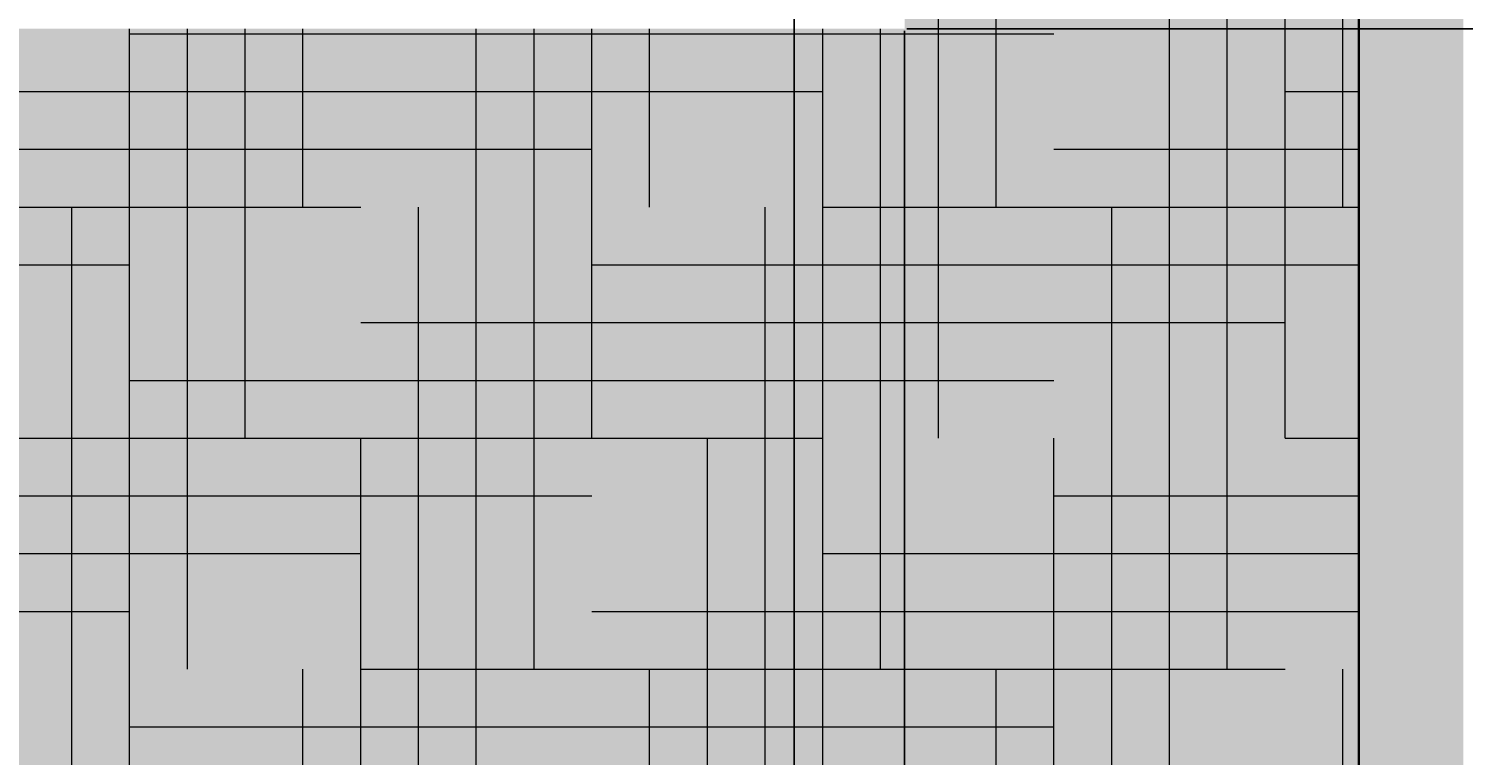
# Model space of a CAD drawing. Units: feet. Extents: x 2695 to 2912, y 795 to 1139.
# Tile 9 of 83: x 2734 to 2774, y 855 to 875. Entities that reach past the tile are written whole.
import ezdxf

# ---------------------------------------------------------------- set-up
doc = ezdxf.new("R2010")
doc.units = ezdxf.units.FT
for name, color, linetype, lineweight in [('A-ANNO-DIMS', 2, 'Continuous', 18), ('A-ELEV', 7, 'Continuous', 35), ('A-ELEV-PATT', 252, 'Continuous', 13)]:
    doc.layers.add(name, color=color, linetype=linetype, lineweight=lineweight)
doc.styles.get("Standard").update_dxf_attribs({"font": 'arial.ttf'})
doc.dimstyles.get("Standard").update_dxf_attribs({"dimtxt": 0.18, "dimasz": 0.18, "dimexe": 0.18, "dimexo": 0.0625, "dimgap": 0.09, "dimtad": 0, "dimtih": 1, "dimtoh": 1, "dimdec": 1, "dimzin": 0, "dimdsep": 46, "dimlunit": 3, "dimtxsty": 'Standard', "dimcen": 0.09, "dimadec": 0, "dimazin": 0, "dimtfac": 1, "dimtdec": 1, "dimtofl": 0, "dimtmove": 0, "dimatfit": 3, "dimfxl": 1, "dimtolj": 1, "dimtzin": 0, "dimarcsym": 0})

# ---------------------------------------------------------------- blocks, each defined once
blk = doc.blocks.new('*D3')
at = {"layer": 'A-ANNO-DIMS', "color": 0, "lineweight": -2, "transparency": 16777216}
for p, q in [((2724.189, 874.795), (2724.189, 794.976)), ((2758.151, 874.795), (2758.151, 794.976)), ((2724.369, 795.156), (2740.777, 795.156)), ((2757.971, 795.156), (2741.564, 795.156))]:
    blk.add_line(p, q, dxfattribs=at)
at = {"layer": 'A-ANNO-DIMS', "color": 0, "transparency": 16777216}
for points in [[(2724.369, 795.186), (2724.369, 795.126), (2724.189, 795.156)], [(2757.971, 795.186), (2757.971, 795.126), (2758.151, 795.156)]]:
    blk.add_solid(points, dxfattribs=at)
at = {"layer": 'Defpoints', "color": 0, "transparency": 16777216}
for p in [(2724.189, 874.857), (2758.151, 874.857), (2758.151, 795.156)]:
    blk.add_point(p, dxfattribs=at)
at = {"layer": 'A-ANNO-DIMS', "color": 0, "transparency": 16777216, "insert": (2741.17, 795.156), "char_height": 0.18, "attachment_point": 5}
blk.add_mtext('\\A1;33.96', dxfattribs=at)
blk = doc.blocks.new('*D4')
at = {"layer": 'A-ANNO-DIMS', "color": 0, "lineweight": -2, "transparency": 16777216}
for p, q in [((2758.151, 874.795), (2758.151, 794.976)), ((2773.503, 810.868), (2773.503, 794.976)), ((2758.331, 795.156), (2765.441, 795.156)), ((2773.323, 795.156), (2766.213, 795.156))]:
    blk.add_line(p, q, dxfattribs=at)
at = {"layer": 'A-ANNO-DIMS', "color": 0, "transparency": 16777216}
for points in [[(2758.331, 795.186), (2758.331, 795.126), (2758.151, 795.156)], [(2773.323, 795.186), (2773.323, 795.126), (2773.503, 795.156)]]:
    blk.add_solid(points, dxfattribs=at)
at = {"layer": 'Defpoints', "color": 0, "transparency": 16777216}
for p in [(2758.151, 874.857), (2773.503, 810.931), (2773.503, 795.156)]:
    blk.add_point(p, dxfattribs=at)
at = {"layer": 'A-ANNO-DIMS', "color": 0, "transparency": 16777216, "insert": (2765.827, 795.156), "char_height": 0.18, "attachment_point": 5}
blk.add_mtext('\\A1;15.35', dxfattribs=at)
blk = doc.blocks.new('*D13')
at = {"layer": 'A-ANNO-DIMS', "color": 0, "lineweight": -2, "transparency": 16777216}
for p, q in [((2758.214, 874.857), (2911.424, 874.857)), ((2911.244, 874.677), (2911.244, 843.076)), ((2911.244, 811.111), (2911.244, 842.712)), ((2890.699, 810.931), (2911.424, 810.931))]:
    blk.add_line(p, q, dxfattribs=at)
at = {"layer": 'A-ANNO-DIMS', "color": 0, "transparency": 16777216}
for points in [[(2911.214, 874.677), (2911.274, 874.677), (2911.244, 874.857)], [(2911.214, 811.111), (2911.274, 811.111), (2911.244, 810.931)]]:
    blk.add_solid(points, dxfattribs=at)
at = {"layer": 'Defpoints', "color": 0, "transparency": 16777216}
for p in [(2758.151, 874.857), (2911.244, 874.857), (2890.636, 810.931)]:
    blk.add_point(p, dxfattribs=at)
at = {"layer": 'A-ANNO-DIMS', "color": 0, "transparency": 16777216, "insert": (2911.244, 842.894), "char_height": 0.18, "attachment_point": 5}
blk.add_mtext('\\A1;63.93', dxfattribs=at)
blk = doc.blocks.new('*D14')
at = {"layer": 'A-ANNO-DIMS', "color": 0, "lineweight": -2, "transparency": 16777216}
for p, q in [((2838.439, 905.514), (2911.424, 905.514)), ((2911.244, 905.334), (2911.244, 890.368)), ((2911.244, 875.037), (2911.244, 890.004)), ((2758.214, 874.857), (2911.424, 874.857))]:
    blk.add_line(p, q, dxfattribs=at)
at = {"layer": 'A-ANNO-DIMS', "color": 0, "transparency": 16777216}
for points in [[(2911.214, 905.334), (2911.274, 905.334), (2911.244, 905.514)], [(2911.214, 875.037), (2911.274, 875.037), (2911.244, 874.857)]]:
    blk.add_solid(points, dxfattribs=at)
at = {"layer": 'Defpoints', "color": 0, "transparency": 16777216}
for p in [(2838.377, 905.514), (2911.244, 905.514), (2758.151, 874.857)]:
    blk.add_point(p, dxfattribs=at)
at = {"layer": 'A-ANNO-DIMS', "color": 0, "transparency": 16777216, "insert": (2911.244, 890.186), "char_height": 0.18, "attachment_point": 5}
blk.add_mtext('\\A1;30.66', dxfattribs=at)
blk = doc.blocks.new('*D24')
at = {"layer": 'A-ANNO-DIMS', "color": 0, "lineweight": -2, "transparency": 16777216}
for p, q in [((2730.708, 936.868), (2730.708, 794.976)), ((2755.112, 936.868), (2755.112, 794.976)), ((2730.888, 795.156), (2742.446, 795.156)), ((2754.932, 795.156), (2743.375, 795.156))]:
    blk.add_line(p, q, dxfattribs=at)
at = {"layer": 'A-ANNO-DIMS', "color": 0, "transparency": 16777216}
for points in [[(2730.888, 795.186), (2730.888, 795.126), (2730.708, 795.156)], [(2754.932, 795.186), (2754.932, 795.126), (2755.112, 795.156)]]:
    blk.add_solid(points, dxfattribs=at)
at = {"layer": 'Defpoints', "color": 0, "transparency": 16777216}
for p in [(2730.708, 936.931), (2755.112, 936.931), (2755.112, 795.156)]:
    blk.add_point(p, dxfattribs=at)
at = {"layer": 'A-ANNO-DIMS', "color": 0, "transparency": 16777216, "insert": (2742.91, 795.156), "char_height": 0.18, "attachment_point": 5}
blk.add_mtext('\\A1;24.404', dxfattribs=at)
blk = doc.blocks.new('*D25')
at = {"layer": 'A-ANNO-DIMS', "color": 0, "lineweight": -2, "transparency": 16777216}
for p, q in [((2755.112, 936.868), (2755.112, 794.976)), ((2770.636, 936.868), (2770.636, 794.976)), ((2755.292, 795.156), (2762.419, 795.156)), ((2770.456, 795.156), (2763.329, 795.156))]:
    blk.add_line(p, q, dxfattribs=at)
at = {"layer": 'A-ANNO-DIMS', "color": 0, "transparency": 16777216}
for points in [[(2755.292, 795.186), (2755.292, 795.126), (2755.112, 795.156)], [(2770.456, 795.186), (2770.456, 795.126), (2770.636, 795.156)]]:
    blk.add_solid(points, dxfattribs=at)
at = {"layer": 'Defpoints', "color": 0, "transparency": 16777216}
for p in [(2755.112, 936.931), (2770.636, 936.931), (2770.636, 795.156)]:
    blk.add_point(p, dxfattribs=at)
at = {"layer": 'A-ANNO-DIMS', "color": 0, "transparency": 16777216, "insert": (2762.874, 795.156), "char_height": 0.18, "attachment_point": 5}
blk.add_mtext('\\A1;15.524', dxfattribs=at)

msp = doc.modelspace()

# ---------------------------------------------------------------- hatches: boundary and pattern name
at = {"layer": 'A-ELEV-PATT'}
h = msp.add_hatch(color=256, dxfattribs=at)
h.set_gradient(color1=(147, 149, 152), color2=(147, 149, 152), tint=1)
h.paths.add_polyline_path([(2770.6361, 1118.4096), (2710.6361, 1118.4096), (2710.6361, 1062.9306), (2770.6361, 1062.9306)])
h.paths.add_polyline_path([(2890.6361, 1103.3378), (2770.6361, 1103.3378), (2770.6361, 1062.9306), (2890.6361, 1062.9306)])
h.paths.add_polyline_path([(2730.7081, 1048.1052), (2755.1125, 1048.1052), (2755.1125, 936.9306), (2770.6361, 936.9306), (2770.6361, 1050.3105), (2715.8852, 1050.3105), (2715.8852, 936.9306), (2730.7081, 936.9306)])
h.paths.add_polyline_path([(2890.6361, 1050.3105), (2770.6361, 1050.3105), (2770.6361, 971.9673), (2778.0341, 971.9673), (2778.0341, 1020.8235), (2843.575, 1020.8235), (2843.575, 971.9673), (2890.6361, 971.9673)])
h.paths.add_polyline_path([(2888.1882, 970.7156), (2843.575, 970.7156), (2843.575, 964.8267), (2888.1882, 964.8267)])
h.paths.add_polyline_path([(2888.1882, 964.1328), (2843.575, 964.1328), (2843.575, 956.614), (2888.1882, 956.614)])
h.paths.add_polyline_path([(2888.1882, 955.9202), (2843.575, 955.9202), (2843.575, 949.2892), (2888.1882, 949.2892)])
h.paths.add_polyline_path([(2888.1882, 948.5954), (2843.575, 948.5954), (2843.575, 941.3507), (2888.1882, 941.3507)])
h.paths.add_polyline_path([(2888.1882, 940.6569), (2843.575, 940.6569), (2843.575, 936.9306), (2888.1882, 936.9306)])
h.paths.add_polyline_path([(2890.6361, 970.7156), (2888.9368, 970.7156), (2888.9368, 964.8267), (2890.6361, 964.8267)])
h.paths.add_polyline_path([(2890.6361, 964.1328), (2888.9368, 964.1328), (2888.9368, 956.614), (2890.6361, 956.614)])
h.paths.add_polyline_path([(2890.6361, 955.9202), (2888.9368, 955.9202), (2888.9368, 949.2892), (2890.6361, 949.2892)])
h.paths.add_polyline_path([(2890.6361, 940.6569), (2888.9368, 940.6569), (2888.9368, 936.9306), (2890.6361, 936.9306)])
h.paths.add_polyline_path([(2890.6361, 948.5954), (2888.9368, 948.5954), (2888.9368, 941.3507), (2890.6361, 941.3507)])
h.paths.add_polyline_path([(2772.5216, 970.7156), (2770.6361, 970.7156), (2770.6361, 964.8267), (2772.5216, 964.8267)])
h.paths.add_polyline_path([(2772.5216, 964.1328), (2770.6361, 964.1328), (2770.6361, 956.614), (2772.5216, 956.614)])
h.paths.add_polyline_path([(2772.5216, 955.9202), (2770.6361, 955.9202), (2770.6361, 949.2892), (2772.5216, 949.2892)])
h.paths.add_polyline_path([(2772.5216, 948.5954), (2770.6361, 948.5954), (2770.6361, 941.3507), (2772.5216, 941.3507)])
h.paths.add_polyline_path([(2772.5216, 940.6569), (2770.6361, 940.6569), (2770.6361, 936.9306), (2772.5216, 936.9306)])
h.paths.add_polyline_path([(2778.0341, 940.6569), (2773.2702, 940.6569), (2773.2702, 936.9306), (2778.0341, 936.9306)])
h.paths.add_polyline_path([(2778.0341, 970.7156), (2773.2702, 970.7156), (2773.2702, 964.8267), (2778.0341, 964.8267)])
h.paths.add_polyline_path([(2778.0341, 964.1328), (2773.2702, 964.1328), (2773.2702, 956.614), (2778.0341, 956.614)])
h.paths.add_polyline_path([(2778.0341, 955.9202), (2773.2702, 955.9202), (2773.2702, 949.2892), (2778.0341, 949.2892)])
h.paths.add_polyline_path([(2778.0341, 948.5954), (2773.2702, 948.5954), (2773.2702, 941.3507), (2778.0341, 941.3507)])
h.paths.add_polyline_path([(2810.0407, 940.6569), (2780.0341, 940.6569), (2780.0341, 936.9306), (2810.0407, 936.9306)])
h.paths.add_polyline_path([(2890.6361, 924.3105), (2770.6361, 924.3105), (2770.6361, 810.9306), (2773.5029, 810.9306), (2773.5029, 905.5143), (2805.9398, 905.5143), (2838.3767, 905.5143), (2838.3767, 810.9306), (2890.6361, 810.9306)])
h = msp.add_hatch(color=256, dxfattribs=at)
h.set_gradient(color1=(255, 255, 255))
h.paths.add_polyline_path([(2770.6361, 924.3105), (2716.5358, 924.3105), (2716.5358, 810.9306), (2770.6361, 810.9306)])
h.paths.add_polyline_path([(2758.1515, 902.577), (2758.1515, 874.8571), (2724.1893, 874.8571), (2724.1893, 902.577)], flags=16)
h.paths.add_polyline_path([(2756.1515, 900.577), (2756.1515, 876.8571), (2726.1893, 876.8571), (2726.1893, 900.577)], flags=0)
h.paths.add_polyline_path([(2740.7302, 900.577), (2741.6105, 900.577), (2741.6105, 876.8571), (2740.7302, 876.8571)], flags=0)
h = msp.add_hatch(dxfattribs=at)
h.set_pattern_fill('HOUND', color=256, style=0)
h.paths.add_polyline_path([(2770.6361, 924.3105), (2716.5358, 924.3105), (2716.5358, 810.9306), (2770.6361, 810.9306)])
h.paths.add_polyline_path([(2724.1893, 874.8571), (2724.1893, 902.577), (2758.1515, 902.577), (2758.1515, 874.8571)], flags=16)
h.paths.add_polyline_path([(2756.1515, 876.8571), (2726.1893, 876.8571), (2726.1893, 900.577), (2756.1515, 900.577)], flags=0)
h.paths.add_polyline_path([(2741.6105, 876.8571), (2740.7302, 876.8571), (2740.7302, 900.577), (2741.6105, 900.577)], flags=0)

# ---------------------------------------------------------------- linework, layer by layer
at = {"layer": 'A-ELEV'}
for p, q in [((2770.6361, 924.3105), (2770.6361, 810.9306)), ((2770.6361, 810.9306), (2770.6361, 924.3105))]:
    msp.add_line(p, q, dxfattribs=at)
msp.add_lwpolyline([(2716.5358, 924.3105), (2770.6361, 924.3105), (2770.6361, 810.9306), (2716.5358, 810.9306)], close=True, dxfattribs=at)

# ---------------------------------------------------------------- dimensions: what is measured, and where the dimension line sits
at = {"layer": 'A-ANNO-DIMS'}
for base, p1, p2, override, picture, middle in [((2755.1125, 795.1556), (2730.7081, 936.9306), (2755.1125, 936.9306), {"dimdec": 3, "dimlfac": 1, "dimrnd": 0, "dimzin": 0, "dimdsep": 46, "dimlunit": 2}, '*D24', (2742.9103, 795.1556)), ((2770.6361, 795.1556), (2755.1125, 936.9306), (2770.6361, 936.9306), {"dimdec": 3, "dimlfac": 1, "dimrnd": 0, "dimzin": 0, "dimdsep": 46, "dimlunit": 2}, '*D25', (2762.8743, 795.1556)), ((2758.1515, 795.1556), (2724.1893, 874.8571), (2758.1515, 874.8571), {"dimdec": 2, "dimlfac": 1, "dimrnd": 0, "dimzin": 0, "dimdsep": 46, "dimlunit": 2}, '*D3', (2741.1704, 795.1556)), ((2773.5029, 795.1556), (2758.1515, 874.8571), (2773.5029, 810.9306), {"dimdec": 2, "dimlfac": 1, "dimrnd": 0, "dimzin": 0, "dimdsep": 46, "dimlunit": 2}, '*D4', (2765.8272, 795.1556))]:
    dim = msp.add_linear_dim(base=base, p1=p1, p2=p2, dimstyle='Standard', override=override, dxfattribs=at)
    dim.commit()
    dim.dimension.update_dxf_attribs({"geometry": picture, "text_midpoint": middle})
for base, p1, p2, picture, middle in [((2911.2444, 905.5143), (2758.1515, 874.8571), (2838.3767, 905.5143), '*D14', (2911.2444, 890.1857)), ((2911.2444, 874.8571), (2890.6361, 810.9306), (2758.1515, 874.8571), '*D13', (2911.2444, 842.8938))]:
    dim = msp.add_linear_dim(base=base, p1=p1, p2=p2, angle=90, dimstyle='Standard', override={"dimdec": 2, "dimlfac": 1, "dimrnd": 0, "dimzin": 0, "dimdsep": 46, "dimlunit": 2}, dxfattribs=at)
    dim.commit()
    dim.dimension.update_dxf_attribs({"geometry": picture, "text_midpoint": middle})

doc.saveas('drawing.dxf')
